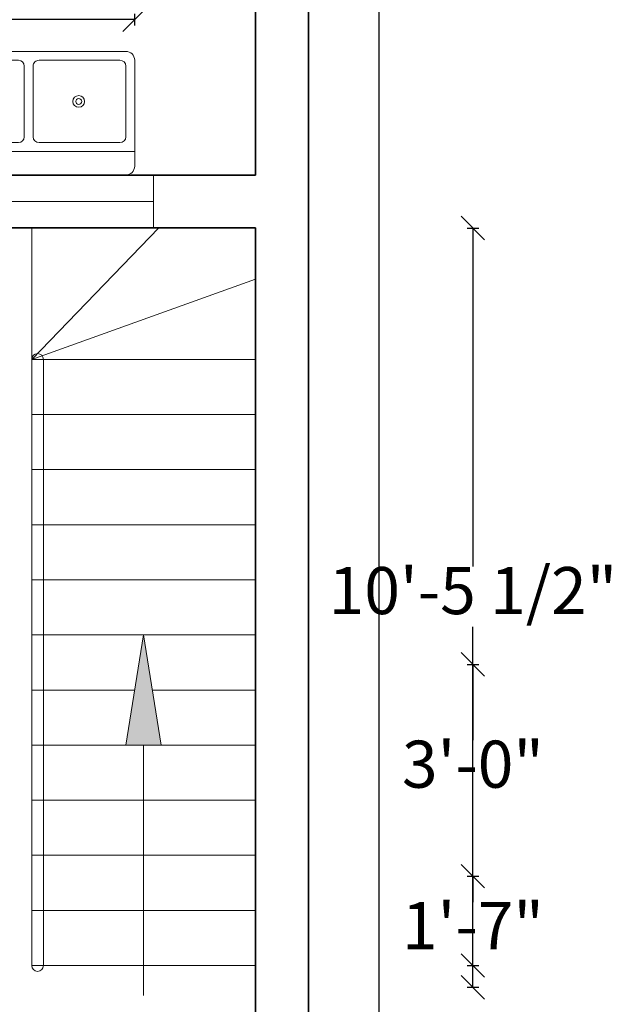
# Model space of a CAD drawing. Units: inches. Extents: x 2558 to 3026, y 433 to 1053.
# Tile 6 of 8: x 2921 to 3021, y 518 to 685. Entities that reach past the tile are written whole.
import ezdxf

# ---------------------------------------------------------------- set-up
doc = ezdxf.new("R2010")
doc.units = ezdxf.units.IN
for name, color, linetype, lineweight in [('A-ANNO-DIMS', 2, 'Continuous', 18), ('A-ANNO-SYMB', 7, 'Continuous', 18), ('A-ANNO-SYMB-PATT', 7, 'Continuous', 13), ('A-FLOR-FIXT', 9, 'Continuous', 18), ('A-FLOR-STRS', 253, 'Continuous', 18), ('A-GLAZ', 5, 'Continuous', 18), ('A-WALL', 7, 'Continuous', 35)]:
    doc.layers.add(name, color=color, linetype=linetype, lineweight=lineweight)
doc.styles.get("Standard").update_dxf_attribs({"font": 'arial.ttf'})
doc.dimstyles.new('ISO-25', dxfattribs={"dimtxt": 8, "dimasz": 4, "dimexe": 1, "dimexo": 1, "dimgap": 1, "dimtad": 0, "dimtih": 1, "dimtoh": 1, "dimlunit": 3, "dimtxsty": 'Standard', "dimblk": 'OBLIQUE', "dimcen": 2.5, "dimclrt": 1, "dimadec": 0, "dimazin": 0, "dimtfac": 1, "dimtmove": 0, "dimatfit": 3, "dimfxl": 1, "dimfxlon": 1, "dimarcsym": 0})

# ---------------------------------------------------------------- blocks, each defined once
blk = doc.blocks.new('Sink-double - 36 in top')
for p, q in [((-18, -4), (18, -4)), ((-0.75, -18.5), (-0.75, -6.5)), ((0.75, -6.5), (0.75, -18.5))]:
    blk.add_line(p, q)
for points in [[(-16.5, 0), (16.5, 0)], [(-18, -19.5), (-18, -1.5)], [(18, -1.5), (18, -19.5)], [(-16.5, -18.5), (-16.5, -6.5)], [(-15.5, -5.5), (-1.75, -5.5)], [(1.75, -5.5), (15.5, -5.5)], [(16.5, -6.5), (16.5, -18.5)], [(-1.75, -19.5), (-15.5, -19.5)], [(15.5, -19.5), (1.75, -19.5)], [(16.5, -21), (-16.5, -21)]]:
    blk.add_lwpolyline(points)
for centre, radius in [((-8.5, -12.5), 1), ((8.5, -12.5), 1), ((-8.5, -12.5), 0.5), ((8.5, -12.5), 0.5)]:
    blk.add_circle(centre, radius)
for centre, radius, start, end in [((-16.5, -1.5), 1.5, 90, 180), ((16.5, -1.5), 1.5, 0, 90), ((-15.5, -6.5), 1, 90, 180), ((-1.75, -6.5), 1, 0, 90), ((1.75, -6.5), 1, 90, 180), ((15.5, -6.5), 1, 0, 90), ((-16.5, -19.5), 1.5, 180, 270), ((-15.5, -18.5), 1, 180, 270), ((-1.75, -18.5), 1, 270, 0), ((1.75, -18.5), 1, 180, 270), ((15.5, -18.5), 1, 270, 0), ((16.5, -19.5), 1.5, 270, 0)]:
    blk.add_arc(centre, radius, start, end)
blk = doc.blocks.new('_Oblique')
at = {"color": 0, "linetype": 'ByBlock', "lineweight": -2}
blk.add_line((-0.5, -0.5), (0.5, 0.5), dxfattribs=at)
blk = doc.blocks.new('*D19')
at = {"layer": 'A-ANNO-DIMS', "color": 0, "lineweight": -2, "transparency": 16777216}
for p, q in [((2980.65, 1012.82), (2982.65, 1012.82)), ((2981.65, 1012.82), (2981.65, 747.89)), ((2981.65, 472.82), (2981.65, 737.76)), ((2980.65, 472.82), (2982.65, 472.82))]:
    blk.add_line(p, q, dxfattribs=at)
at = {"layer": 'Defpoints', "color": 0, "transparency": 16777216}
for p in [(2969.63, 1012.82), (2969.63, 472.82), (2981.65, 472.82)]:
    blk.add_point(p, dxfattribs=at)
at = {"layer": 'A-ANNO-DIMS', "color": 0, "lineweight": -2, "transparency": 16777216, "xscale": 4, "yscale": 4, "zscale": 4}
for p, rotation in [((2981.65, 1012.82), 90), ((2981.65, 472.82), 270)]:
    blk.add_blockref('_Oblique', p, dxfattribs=dict(at, rotation=rotation))
at = {"layer": 'A-ANNO-DIMS', "color": 0, "transparency": 16777216, "insert": (2981.65, 742.82), "char_height": 8, "attachment_point": 5}
blk.add_mtext("45'", dxfattribs=at)
blk = doc.blocks.new('*D41')
at = {"layer": 'A-ANNO-DIMS', "color": 0, "lineweight": -2, "transparency": 16777216}
for p, q in [((2904.13, 684.22), (2904.13, 686.22)), ((2940.13, 684.22), (2940.13, 686.22)), ((2904.13, 685.22), (2900.13, 685.22)), ((2940.13, 685.22), (2904.13, 685.22))]:
    blk.add_line(p, q, dxfattribs=at)
at = {"layer": 'Defpoints', "color": 0, "transparency": 16777216}
for p in [(2904.13, 685.22), (2904.13, 679.82), (2940.13, 679.82)]:
    blk.add_point(p, dxfattribs=at)
at = {"layer": 'A-ANNO-DIMS', "color": 0, "lineweight": -2, "transparency": 16777216, "xscale": 4, "yscale": 4, "zscale": 4, "rotation": 180}
blk.add_blockref('_Oblique', (2904.13, 685.22), dxfattribs=at)
at = {"layer": 'A-ANNO-DIMS', "color": 0, "lineweight": -2, "transparency": 16777216, "xscale": 4, "yscale": 4, "zscale": 4}
blk.add_blockref('_Oblique', (2940.13, 685.22), dxfattribs=at)
at = {"layer": 'A-ANNO-DIMS', "color": 1, "transparency": 16777216, "insert": (2873.92, 685.22), "char_height": 8, "attachment_point": 5}
blk.add_mtext('SINK 3\'-0"', dxfattribs=at)
blk = doc.blocks.new('*D46')
at = {"layer": 'A-ANNO-DIMS', "color": 0, "lineweight": -2, "transparency": 16777216}
for p, q in [((2922.63, 445.87), (2922.63, 443.87)), ((2960.63, 445.87), (2960.63, 443.87)), ((2922.63, 444.87), (2930, 444.87)), ((2960.63, 444.87), (2953.26, 444.87))]:
    blk.add_line(p, q, dxfattribs=at)
at = {"layer": 'Defpoints', "color": 0, "transparency": 16777216}
for p in [(2922.63, 524.53), (2960.63, 524.53), (2960.63, 444.87)]:
    blk.add_point(p, dxfattribs=at)
at = {"layer": 'A-ANNO-DIMS', "color": 0, "lineweight": -2, "transparency": 16777216, "xscale": 4, "yscale": 4, "zscale": 4, "rotation": 180}
blk.add_blockref('_Oblique', (2922.63, 444.87), dxfattribs=at)
at = {"layer": 'A-ANNO-DIMS', "color": 0, "lineweight": -2, "transparency": 16777216, "xscale": 4, "yscale": 4, "zscale": 4}
blk.add_blockref('_Oblique', (2960.63, 444.87), dxfattribs=at)
at = {"layer": 'A-ANNO-DIMS', "color": 1, "transparency": 16777216, "insert": (2941.63, 444.87), "char_height": 8, "attachment_point": 5}
blk.add_mtext('3\'-2"', dxfattribs=at)
blk = doc.blocks.new('*D47')
at = {"layer": 'A-ANNO-DIMS', "color": 0, "lineweight": -2, "transparency": 16777216}
for p, q in [((2996.58, 649.82), (2998.58, 649.82)), ((2997.58, 649.82), (2997.58, 592.31)), ((2997.58, 524.53), (2997.58, 582.04)), ((2996.58, 524.53), (2998.58, 524.53))]:
    blk.add_line(p, q, dxfattribs=at)
at = {"layer": 'Defpoints', "color": 0, "transparency": 16777216}
for p in [(2960.63, 649.82), (2960.63, 524.53), (2997.58, 524.53)]:
    blk.add_point(p, dxfattribs=at)
at = {"layer": 'A-ANNO-DIMS', "color": 0, "lineweight": -2, "transparency": 16777216, "xscale": 4, "yscale": 4, "zscale": 4}
for p, rotation in [((2997.58, 649.82), 90), ((2997.58, 524.53), 270)]:
    blk.add_blockref('_Oblique', p, dxfattribs=dict(at, rotation=rotation))
at = {"layer": 'A-ANNO-DIMS', "color": 1, "transparency": 16777216, "insert": (2997.58, 587.18), "char_height": 8, "attachment_point": 5}
blk.add_mtext('10\'-5 1/2"', dxfattribs=at)
blk = doc.blocks.new('*D58')
at = {"layer": 'A-ANNO-DIMS', "color": 0, "lineweight": -2, "transparency": 16777216}
for p, q in [((2901.29, 1039.77), (2901.29, 1041.77)), ((2901.29, 1040.77), (2910.69, 1040.77)), ((2943.34, 1040.77), (2933.95, 1040.77)), ((2943.34, 1039.77), (2943.34, 1041.77))]:
    blk.add_line(p, q, dxfattribs=at)
at = {"layer": 'Defpoints', "color": 0, "transparency": 16777216}
for p in [(2943.34, 1040.77), (2901.29, 649.82), (2943.34, 649.82)]:
    blk.add_point(p, dxfattribs=at)
at = {"layer": 'A-ANNO-DIMS', "color": 0, "lineweight": -2, "transparency": 16777216, "xscale": 4, "yscale": 4, "zscale": 4, "rotation": 180}
blk.add_blockref('_Oblique', (2901.29, 1040.77), dxfattribs=at)
at = {"layer": 'A-ANNO-DIMS', "color": 0, "lineweight": -2, "transparency": 16777216, "xscale": 4, "yscale": 4, "zscale": 4}
blk.add_blockref('_Oblique', (2943.34, 1040.77), dxfattribs=at)
at = {"layer": 'A-ANNO-DIMS', "color": 1, "transparency": 16777216, "insert": (2922.32, 1040.77), "char_height": 8, "attachment_point": 5}
blk.add_mtext('3\'-6"', dxfattribs=at)
blk = doc.blocks.new('*D60')
at = {"layer": 'A-ANNO-DIMS', "color": 0, "lineweight": -2, "transparency": 16777216}
for p, q in [((2996.58, 575.69), (2998.58, 575.69)), ((2997.58, 575.69), (2997.58, 562.78)), ((2997.58, 539.69), (2997.58, 552.6)), ((2996.58, 539.69), (2998.58, 539.69))]:
    blk.add_line(p, q, dxfattribs=at)
at = {"layer": 'Defpoints', "color": 0, "transparency": 16777216}
for p in [(2807.63, 575.69), (2997.58, 575.69), (2807.63, 539.69)]:
    blk.add_point(p, dxfattribs=at)
at = {"layer": 'A-ANNO-DIMS', "color": 0, "lineweight": -2, "transparency": 16777216, "xscale": 4, "yscale": 4, "zscale": 4}
for p, rotation in [((2997.58, 575.69), 90), ((2997.58, 539.69), 270)]:
    blk.add_blockref('_Oblique', p, dxfattribs=dict(at, rotation=rotation))
at = {"layer": 'A-ANNO-DIMS', "color": 1, "transparency": 16777216, "insert": (2997.58, 557.69), "char_height": 8, "attachment_point": 5}
blk.add_mtext('3\'-0"', dxfattribs=at)
blk = doc.blocks.new('*D71')
at = {"layer": 'A-ANNO-DIMS', "color": 0, "lineweight": -2, "transparency": 16777216}
for p, q in [((2996.58, 539.69), (2998.58, 539.69)), ((2997.58, 539.69), (2997.58, 535.27)), ((2997.58, 520.82), (2997.58, 525.24)), ((2996.58, 520.82), (2998.58, 520.82))]:
    blk.add_line(p, q, dxfattribs=at)
at = {"layer": 'Defpoints', "color": 0, "transparency": 16777216}
for p in [(2807.63, 539.69), (2997.58, 539.69), (2807.63, 520.82)]:
    blk.add_point(p, dxfattribs=at)
at = {"layer": 'A-ANNO-DIMS', "color": 0, "lineweight": -2, "transparency": 16777216, "xscale": 4, "yscale": 4, "zscale": 4}
for p, rotation in [((2997.58, 539.69), 90), ((2997.58, 520.82), 270)]:
    blk.add_blockref('_Oblique', p, dxfattribs=dict(at, rotation=rotation))
at = {"layer": 'A-ANNO-DIMS', "color": 1, "transparency": 16777216, "insert": (2997.58, 530.26), "char_height": 8, "attachment_point": 5}
blk.add_mtext('1\'-7"', dxfattribs=at)
blk = doc.blocks.new('*D73')
at = {"layer": 'A-ANNO-DIMS', "color": 0, "lineweight": -2, "transparency": 16777216}
for p, q in [((2816.63, 1039.77), (2816.63, 1041.77)), ((2816.63, 1040.77), (2870.66, 1040.77)), ((2959.63, 1040.77), (2905.6, 1040.77)), ((2959.63, 1039.77), (2959.63, 1041.77))]:
    blk.add_line(p, q, dxfattribs=at)
at = {"layer": 'Defpoints', "color": 0, "transparency": 16777216}
for p in [(2959.63, 1040.77), (2816.63, 481.83), (2959.63, 481.82)]:
    blk.add_point(p, dxfattribs=at)
at = {"layer": 'A-ANNO-DIMS', "color": 0, "lineweight": -2, "transparency": 16777216, "xscale": 4, "yscale": 4, "zscale": 4, "rotation": 180}
blk.add_blockref('_Oblique', (2816.63, 1040.77), dxfattribs=at)
at = {"layer": 'A-ANNO-DIMS', "color": 0, "lineweight": -2, "transparency": 16777216, "xscale": 4, "yscale": 4, "zscale": 4}
blk.add_blockref('_Oblique', (2959.63, 1040.77), dxfattribs=at)
at = {"layer": 'A-ANNO-DIMS', "color": 1, "transparency": 16777216, "insert": (2888.13, 1040.77), "char_height": 8, "attachment_point": 5}
blk.add_mtext('11\'-11"', dxfattribs=at)

msp = doc.modelspace()

# ---------------------------------------------------------------- hatches: boundary and pattern name
at = {"layer": 'A-ANNO-SYMB-PATT'}
h = msp.add_hatch(color=256, dxfattribs=at)
h.dxf.hatch_style = 1
h.paths.add_polyline_path([(2941.633, 580.687), (2938.633, 561.966), (2944.633, 561.966)])

# ---------------------------------------------------------------- linework, layer by layer
at = {"layer": 'A-ANNO-SYMB'}
for p, q in [((2938.633, 561.966), (2941.633, 580.687)), ((2944.633, 561.966), (2941.633, 580.687)), ((2944.633, 561.966), (2938.633, 561.966)), ((2941.633, 519.427), (2941.633, 561.966))]:
    msp.add_line(p, q, dxfattribs=at)
at = {"layer": 'A-FLOR-STRS'}
for p, q in [((2922.633, 524.526), (2922.633, 649.825)), ((2922.633, 627.487), (2944.261, 649.825)), ((2922.633, 627.487), (2960.633, 641.133)), ((2960.633, 627.487), (2922.633, 627.487)), ((2924.633, 524.526), (2924.633, 627.487)), ((2960.633, 618.127), (2922.633, 618.127)), ((2960.633, 608.767), (2922.633, 608.767)), ((2960.633, 599.407), (2922.633, 599.407)), ((2960.633, 590.047), (2922.633, 590.047)), ((2960.633, 580.687), (2922.633, 580.687)), ((2940.133, 571.326), (2922.633, 571.326)), ((2960.633, 571.326), (2943.133, 571.326)), ((2938.633, 561.966), (2922.633, 561.966)), ((2960.633, 561.966), (2944.633, 561.966)), ((2960.633, 552.606), (2922.633, 552.606)), ((2960.633, 543.246), (2922.633, 543.246)), ((2960.633, 533.886), (2922.633, 533.886)), ((2960.633, 524.526), (2922.633, 524.526))]:
    msp.add_line(p, q, dxfattribs=at)
for centre, start, end in [((2923.633, 627.487), 0, 180), ((2923.633, 524.526), 180, 0)]:
    msp.add_arc(centre, 1, start, end, dxfattribs=at)
at = {"layer": 'A-GLAZ'}
for p, q in [((2943.344, 658.825), (2943.344, 649.825)), ((2901.294, 654.325), (2943.344, 654.325))]:
    msp.add_line(p, q, dxfattribs=at)
at = {"layer": 'A-WALL'}
for p, q in [((2969.633, 472.825), (2969.633, 1012.825)), ((2960.633, 658.825), (2960.633, 790.825)), ((2960.633, 658.825), (2881.133, 658.825)), ((2960.633, 649.825), (2867.633, 649.825)), ((2960.633, 481.825), (2960.633, 649.825))]:
    msp.add_line(p, q, dxfattribs=at)

# ---------------------------------------------------------------- block references
at = {"layer": 'A-FLOR-FIXT', "rotation": 180}
msp.add_blockref('Sink-double - 36 in top', (2922.13, 658.825), dxfattribs=at)

# ---------------------------------------------------------------- dimensions: what is measured, and where the dimension line sits
at = {"layer": 'A-ANNO-DIMS'}
for base, p1, p2, picture, middle in [((2959.633, 1040.775), (2816.633, 481.827), (2959.633, 481.825), '*D73', (2888.133, 1040.775)), ((2943.3439, 1040.7746), (2901.2944, 649.8246), (2943.3439, 649.8246), '*D58', (2922.3191, 1040.7746)), ((2960.633, 444.875), (2922.633, 524.526), (2960.633, 524.526), '*D46', (2941.633, 444.875))]:
    dim = msp.add_linear_dim(base=base, p1=p1, p2=p2, dimstyle='ISO-25', override={"dimdec": 1, "dimlfac": 1, "dimrnd": 0, "dimzin": 1, "dimdsep": 46, "dimlunit": 4, "dimfrac": 2}, dxfattribs=at)
    dim.commit()
    dim.dimension.update_dxf_attribs({"geometry": picture, "text_midpoint": middle})
for base, p1, p2, override, picture, middle in [((2981.646, 472.825), (2969.633, 1012.825), (2969.633, 472.825), {"dimclrd": 0, "dimclre": 0, "dimclrt": 0}, '*D19', (2981.646, 742.825)), ((2997.583, 524.526), (2960.633, 649.825), (2960.633, 524.526), {"dimdec": 1, "dimlfac": 1, "dimrnd": 0, "dimzin": 1, "dimdsep": 46, "dimlunit": 4, "dimfrac": 2}, '*D47', (2997.583, 587.175)), ((2997.583, 575.691), (2807.633, 539.691), (2807.633, 575.691), {"dimdec": 1, "dimlfac": 1, "dimrnd": 0, "dimzin": 1, "dimdsep": 46, "dimlunit": 4, "dimfrac": 2}, '*D60', (2997.583, 557.691)), ((2997.583, 539.691), (2807.633, 520.825), (2807.633, 539.691), {"dimdec": 1, "dimlfac": 1, "dimrnd": 0, "dimzin": 1, "dimdsep": 46, "dimlunit": 4, "dimfrac": 2}, '*D71', (2997.583, 530.258))]:
    dim = msp.add_linear_dim(base=base, p1=p1, p2=p2, angle=90, dimstyle='ISO-25', override=override, dxfattribs=at)
    dim.commit()
    dim.dimension.update_dxf_attribs({"geometry": picture, "text_midpoint": middle})
dim = msp.add_linear_dim(base=(2904.13, 685.225), p1=(2940.13, 679.825), p2=(2904.13, 679.825), angle=180, text='SINK <>', dimstyle='ISO-25', override={"dimdec": 1, "dimlfac": 1, "dimrnd": 0, "dimzin": 1, "dimdsep": 46, "dimlunit": 4, "dimfrac": 2}, dxfattribs=at)
dim.commit()
dim.dimension.update_dxf_attribs({"geometry": '*D41', "text_midpoint": (2873.922, 685.225)})

doc.saveas('drawing.dxf')
